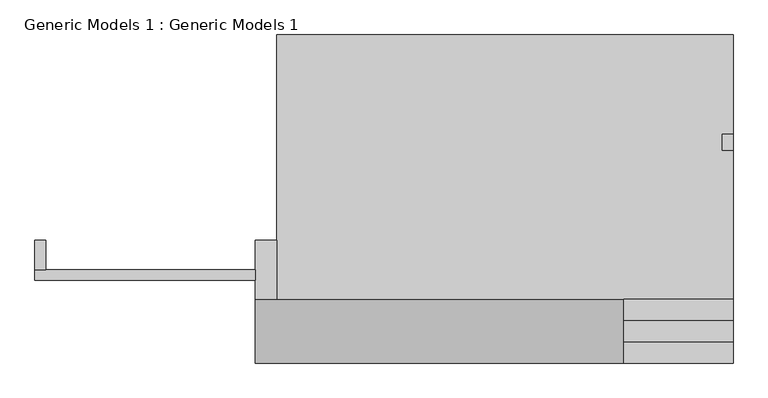
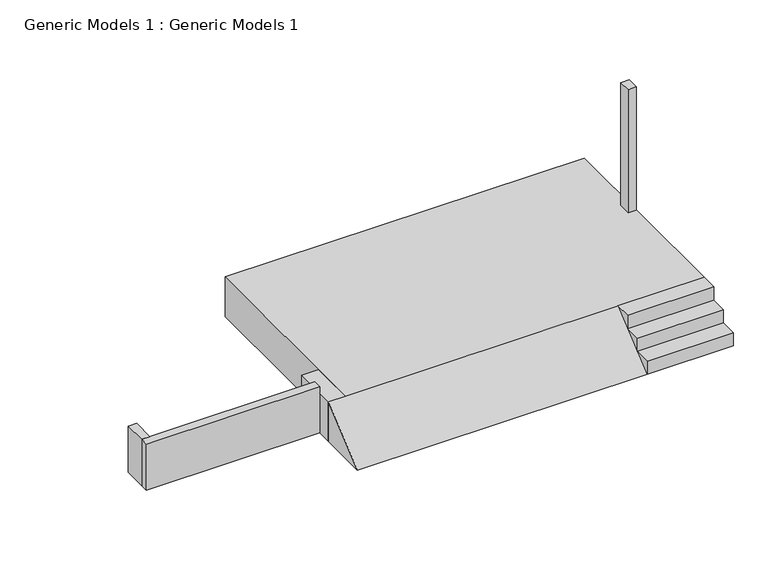
"""IFC4 building model written with IfcOpenShell, lengths in millimetres: proxy geometry, Generic Models 1 : Generic Models 1."""

from ifc_helpers import new_model, si_unit, frame, origin, place, context, project, spatial, polyline, outline, extrude, source, transform, mapped, element, save


def generic_models_1_generic_models_1_9d6986c9(model_context):
    return source(origin(), model_context, "Body", "SweptSolid", [
        extrude(outline(polyline([(-1555.8932179, -152.4), (-641.4932179, 609.6), (-641.4932179, -152.4), (-1555.8932179, -152.4)])), frame((-4692.5540309, 0.0, 0.0), z_axis=(1.0, 0.0, 0.0), x_axis=(0.0, 1.0, 0.0)), (0.0, 0.0, 1.0), 5257.8),
        extrude(outline(polyline([(-641.4932179, -152.4), (-1555.8932179, -152.4), (-1555.8932179, 101.6), (-1251.0932179, 101.6), (-1251.0932179, 355.6), (-946.2932179, 355.6), (-946.2932179, 609.6), (-641.4932179, 609.6), (-641.4932179, -152.4)])), frame((565.2459691, 0.0, 0.0), z_axis=(1.0, 0.0, 0.0), x_axis=(0.0, 1.0, 0.0)), (0.0, 0.0, 1.0), 1562.1),
        extrude(outline(polyline([(1974.9459691, 1481.3177926), (1974.9459691, 1709.9177926), (2127.3459691, 1709.9177926), (2127.3459691, 1481.3177926), (1974.9459691, 1481.3177926)])), frame((0.0, 0.0, 609.6), z_axis=(0.0, 0.0, 1.0), x_axis=(1.0, 0.0, 0.0)), (0.0, 0.0, 1.0), 2362.2),
        extrude(outline(polyline([(-7840.4748309, 195.2033856), (-7688.0748309, 195.2033856), (-7688.0748309, -223.1449161), (-7840.4748309, -223.1449161), (-7840.4748309, 195.2033856)])), frame((0.0, 0.0, -152.4), z_axis=(0.0, 0.0, 1.0), x_axis=(1.0, 0.0, 0.0)), (0.0, 0.0, 1.0), 885.5770356),
        extrude(outline(polyline([(-7840.4748309, -375.8442733), (-7840.4748309, -223.1449161), (-4692.5540309, -223.1449161), (-4692.5540309, -375.8442733), (-7840.4748309, -375.8442733)])), frame((0.0, 0.0, -152.4), z_axis=(0.0, 0.0, 1.0), x_axis=(1.0, 0.0, 0.0)), (0.0, 0.0, 1.0), 885.5770356),
        extrude(outline(polyline([(-4692.5540309, -641.4932179), (-4692.5540309, 195.2033856), (-4387.7540309, 195.2033856), (-4387.7540309, -641.4932179), (-4692.5540309, -641.4932179)])), frame((0.0, 0.0, -152.4), z_axis=(0.0, 0.0, 1.0), x_axis=(1.0, 0.0, 0.0)), (0.0, 0.0, 1.0), 762.0),
        extrude(outline(polyline([(2127.3459691, -641.4932179), (-4387.7540309, -641.4932179), (-4387.7540309, 3128.9033856), (2127.3459691, 3128.9033856), (2127.3459691, -641.4932179)])), frame((0.0, 0.0, -152.4), z_axis=(0.0, 0.0, 1.0), x_axis=(1.0, 0.0, 0.0)), (0.0, 0.0, 1.0), 762.0),
    ])


if __name__ == "__main__":
    model = new_model("IFC4")
    model_context = context("Model", 3, world=origin())
    ifc_project = project(units=[si_unit("LENGTHUNIT", "METRE", prefix="MILLI")], contexts=[model_context])
    site = spatial("IfcSite", under=ifc_project)
    building = spatial("IfcBuilding", under=site)
    placement = place(None, origin())
    generic_models_1_generic_models_1_shape = generic_models_1_generic_models_1_9d6986c9(model_context)
    element("IfcBuildingElementProxy", 1, Name="Generic Models 1 : Generic Models 1", ObjectType="Generic Models 1 : Generic Models 1", at=placement, inside=building, context=model_context, shape_type="MappedRepresentation", body=[
        mapped(generic_models_1_generic_models_1_shape, transform((0.0, 0.0, 0.0), x_axis=(1.0, 0.0, 0.0), y_axis=(0.0, 1.0, 0.0), z_axis=(0.0, 0.0, 1.0))),
    ])
    save(model, "model.ifc")

# Revit data of these elements
# Element 1 (IfcBuildingElementProxy, "Generic Models 1 : Generic Models 1")
#   Materials on its faces: "Gypsum Wall Board", "Gravel"
# Materials
#   "Gypsum Wall Board": class "Generic", colour RGB 127 127 127, transparency 0, Description = "Gypsum Wall Board", Cost = 0
#   "Gravel": class "Generic", colour RGB 120 120 120, transparency 0, Description = "Crushed stone or gravel", Cost = 0
